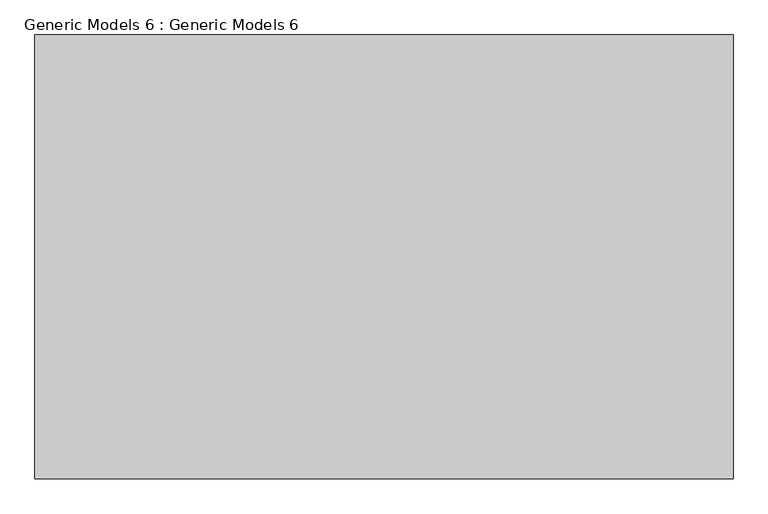
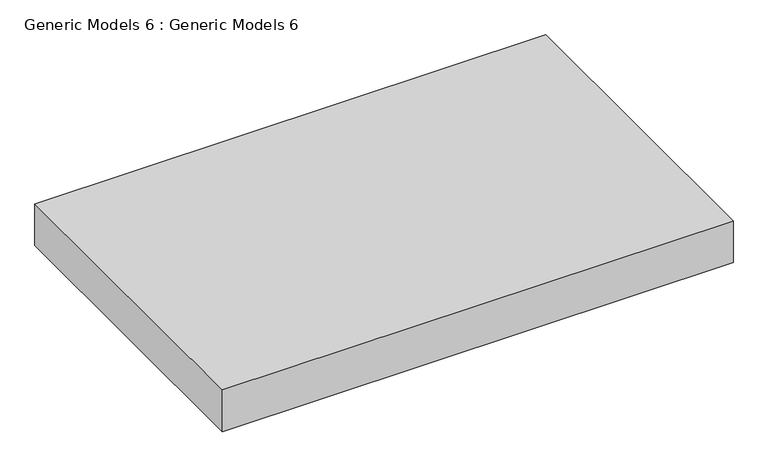
"""IFC4 building model written with IfcOpenShell, lengths in millimetres: proxy geometry, Generic Models 6 : Generic Models 6."""

from ifc_helpers import new_model, si_unit, frame, origin, place, context, project, spatial, polyline, outline, extrude, source, transform, mapped, element, save


def generic_models_6_generic_models_6_f9bdd1e7(model_context):
    return source(origin(), model_context, "Body", "SweptSolid", [
        extrude(outline(polyline([(-15877.1321088, -8905.1468404), (-15877.1321088, -5738.2962979), (-10894.660896, -5738.2962979), (-10894.660896, -8905.1468404), (-15877.1321088, -8905.1468404)])), frame((0.0, 0.0, 10988.8045332), z_axis=(0.0, 0.0, 1.0), x_axis=(1.0, 0.0, 0.0)), (0.0, 0.0, 1.0), 431.8),
    ])


if __name__ == "__main__":
    model = new_model("IFC4")
    model_context = context("Model", 3, world=origin())
    ifc_project = project(units=[si_unit("LENGTHUNIT", "METRE", prefix="MILLI")], contexts=[model_context])
    site = spatial("IfcSite", under=ifc_project)
    building = spatial("IfcBuilding", under=site)
    placement = place(None, origin())
    generic_models_6_generic_models_6_shape = generic_models_6_generic_models_6_f9bdd1e7(model_context)
    element("IfcBuildingElementProxy", 1, Name="Generic Models 6 : Generic Models 6", ObjectType="Generic Models 6 : Generic Models 6", at=placement, inside=building, context=model_context, shape_type="MappedRepresentation", body=[
        mapped(generic_models_6_generic_models_6_shape, transform((0.0, 0.0, 0.0), x_axis=(1.0, 0.0, 0.0), y_axis=(0.0, 1.0, 0.0), z_axis=(0.0, 0.0, 1.0))),
    ])
    save(model, "model.ifc")
